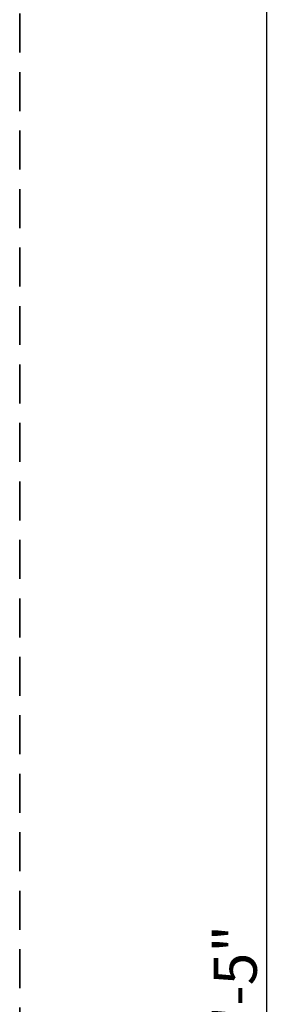
# Model space of a CAD drawing. Units: inches. Extents: x -7 to 1228, y -146 to 1091.
# Tile 85 of 88: x 1187 to 1228, y 531 to 691. Entities that reach past the tile are written whole.
import ezdxf

# ---------------------------------------------------------------- set-up
doc = ezdxf.new("R2010")
doc.units = ezdxf.units.IN
doc.linetypes.add('DASHED2', pattern=[9.525, 6.35, -3.175])
doc.layers.add('A-ANNO-DIMS', color=2, linetype='Continuous', lineweight=18)
doc.layers.add('C-PROP', color=1, linetype='DASHED2', lineweight=35)
doc.styles.get("Standard").update_dxf_attribs({"font": 'arial.ttf'})
doc.dimstyles.new('ISO-25', dxfattribs={"dimtxt": 7, "dimasz": 4, "dimexe": 1.25, "dimexo": 0.625, "dimtad": 1, "dimdec": 1, "dimlunit": 3, "dimtxsty": 'Standard', "dimcen": 2.5, "dimadec": 0, "dimazin": 0, "dimtfac": 1, "dimtdec": 1, "dimtmove": 1, "dimatfit": 3, "dimfxl": 1, "dimarcsym": 0})

# ---------------------------------------------------------------- blocks, each defined once
blk = doc.blocks.new('*D12')
at = {"layer": 'A-ANNO-DIMS', "color": 0, "lineweight": -2, "transparency": 16777216}
for p, q in [((1187.62, 1061), (1228.45, 1061)), ((1227.2, 1057), (1227.2, 4)), ((1187.62, 0), (1228.45, 0))]:
    blk.add_line(p, q, dxfattribs=at)
at = {"layer": 'A-ANNO-DIMS', "color": 0, "transparency": 16777216}
for points in [[(1226.53, 1057), (1227.86, 1057), (1227.2, 1061)], [(1226.53, 4), (1227.86, 4), (1227.2, 0)]]:
    blk.add_solid(points, dxfattribs=at)
at = {"layer": 'Defpoints', "color": 0, "transparency": 16777216}
for p in [(1187, 1061), (1187, 0), (1227.2, 0)]:
    blk.add_point(p, dxfattribs=at)
at = {"layer": 'A-ANNO-DIMS', "color": 0, "transparency": 16777216, "insert": (1223, 530.5), "char_height": 7, "attachment_point": 5, "rotation": 90}
blk.add_mtext('88\'-5"', dxfattribs=at)

msp = doc.modelspace()

# ---------------------------------------------------------------- linework, layer by layer
at = {"layer": 'C-PROP'}
msp.add_line((1187, 0), (1187, 1061), dxfattribs=at)

# ---------------------------------------------------------------- dimensions: what is measured, and where the dimension line sits
at = {"layer": 'A-ANNO-DIMS'}
dim = msp.add_linear_dim(base=(1227.2, 0), p1=(1187, 1061), p2=(1187, 0), angle=90, dimstyle='ISO-25', override={"dimclrd": 0, "dimclre": 0, "dimclrt": 0}, dxfattribs=at)
dim.commit()
dim.dimension.update_dxf_attribs({"geometry": '*D12', "text_midpoint": (1223, 530.5)})

doc.saveas('drawing.dxf')
